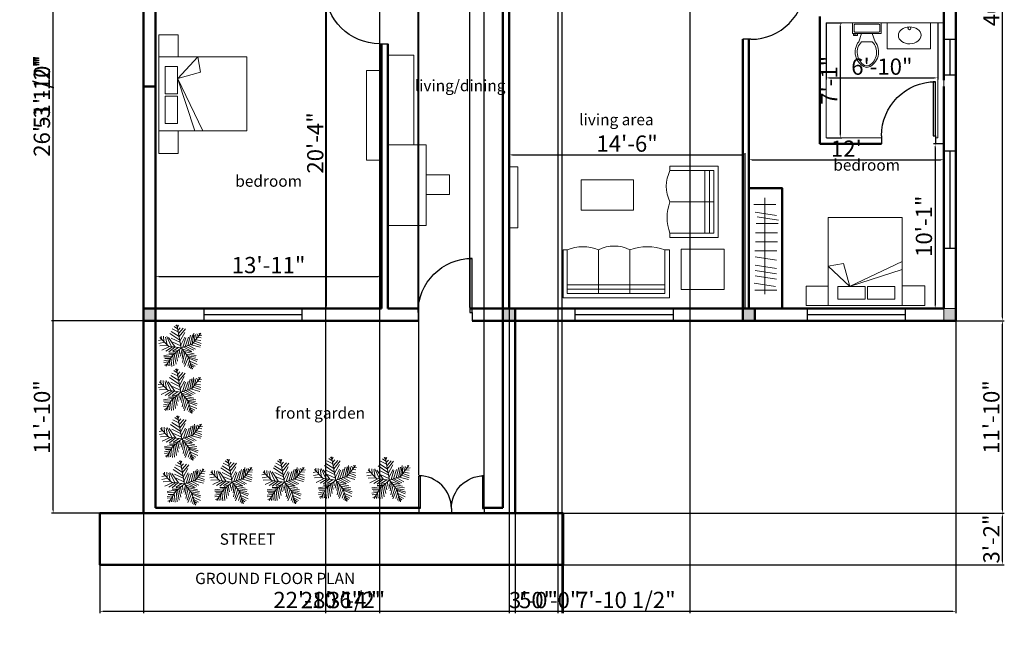
# Model space of a CAD drawing. Units: inches. Extents: x 1367 to 2309, y 1406 to 3826.
# Tile 1 of 9: x 1417 to 2144, y 1406 to 1853. Entities that reach past the tile are written whole.
import ezdxf

# ---------------------------------------------------------------- set-up
doc = ezdxf.new("R2010")
doc.units = ezdxf.units.IN
for name, color, linetype, lineweight in [('A-ANNO-DIMS', 2, 'Continuous', 18), ('A-ANNO-TEXT', 7, 'Continuous', 25), ('A-AREA-IDEN', 3, 'Continuous', 18), ('A-DOOR', 4, 'Continuous', 25), ('A-FLOR-FIXT', 8, 'Continuous', 18), ('A-FURN', 8, 'Continuous', 18), ('A-GLAZ', 4, 'Continuous', 25), ('A-WALL', 7, 'Continuous', 50), ('A-WALL-PATT', 8, 'Continuous', 18), ('garden', 80, 'Continuous', 18)]:
    doc.layers.add(name, color=color, linetype=linetype, lineweight=lineweight)
doc.styles.get("Standard").update_dxf_attribs({"font": 'arial.ttf'})
doc.dimstyles.new('ISO-25', dxfattribs={"dimtxt": 12, "dimasz": 2.5, "dimexe": 1.25, "dimexo": 0.625, "dimtad": 1, "dimdec": 0, "dimlunit": 4, "dimtxsty": 'Standard', "dimcen": 2.5, "dimadec": 0, "dimazin": 0, "dimtfac": 1, "dimtdec": 0, "dimtmove": 0, "dimatfit": 3, "dimfxl": 1, "dimarcsym": 0})

# ---------------------------------------------------------------- blocks, each defined once
blk = doc.blocks.new('*U2')
for p, q in [((0, 0), (0, -6)), ((40, 0), (40, -6))]:
    blk.add_line(p, q)
blk.add_lwpolyline([(0, 0), (0, 40), (1.75, 40), (1.75, 0)], close=True)
blk.add_arc((0, 0), 40, 0, 90)
blk = doc.blocks.new('*U4')
for p, q in [((9.5, -6), (9.5, -2)), ((-10, -8.5), (-8, -8.5)), ((-10, -9.5), (-10, -8.5)), ((-7, -9.5), (-10, -9.5)), ((-8, -8.5), (-8, -8)), ((-7, -8), (-7, -9.5)), ((-4, -8), (-6, -14)), ((4, -14), (-4, -14)), ((4, -8), (6, -14))]:
    blk.add_line(p, q)
blk.add_lwpolyline([(10.5, -8), (10.5, 0), (-10.5, 0), (-10.5, -8)], close=True)
for points in [[(-9.5, -2), (-9.5, -6)], [(8.5, -1), (-8.5, -1)], [(-8.5, -7), (8.5, -7)]]:
    blk.add_lwpolyline(points)
for centre, radius, start, end in [((-8.62, -1.88), 0.884, 81.8699, 188.1301), ((-8.62, -6.12), 0.884, 171.8699, 278.1301), ((8.62, -1.88), 0.884, 351.8699, 98.1301), ((8.62, -6.12), 0.884, 261.8699, 8.1301), ((3.52, -21.58), 12.17, 141.46911, 247.97143), ((4.2, -21.82), 11.33, 136.36773, 238.94682), ((-3.52, -21.58), 12.17, 292.02843, 38.53071), ((-4.2, -21.82), 11.33, 301.05301, 43.63209), ((0, -27.88), 4, 245.73182, 294.26817), ((0, -29), 4, 254.86053, 285.13947)]:
    blk.add_arc(centre, radius, start, end)
blk = doc.blocks.new('*U6')
for p, q in [((-8.737, 47.138), (-17.069, 52.711)), ((-10.186, 53.64), (-13.084, 55.962)), ((0, 0), (-10.5, 57)), ((-9.099, 51.782), (-6.563, 55.962)), ((-7.65, 43.423), (-2.578, 49.46)), ((-31.5, 4.5), (-52.5, 25.5)), ((-48.585, 21.131), (-49.309, 29.026)), ((-43.513, 28.561), (-42.427, 15.558)), ((-38.442, 26.239), (-34.819, 7.663)), ((-35.544, 28.097), (-24.314, 3.947)), ((-14.533, 2.09), (-30.834, 25.31)), ((-3.665, 19.273), (-27.574, 35.527)), ((-5.114, 28.097), (-24.676, 40.636)), ((-7.288, 39.707), (-21.778, 46.673)), ((-5.839, 35.992), (4.667, 48.067)), ((-5.114, 27.632), (10.463, 46.673)), ((-2.941, 16.486), (8.652, 37.85)), ((-1.129, 6.734), (9.014, 26.704)), ((3.942, 1.625), (11.187, 24.381)), ((10.101, 3.483), (17.708, 26.239)), ((16.259, 5.805), (23.142, 31.348)), ((22.055, 7.198), (27.489, 32.277)), ((27, 9), (48, 36)), ((27.127, 9.056), (31.112, 35.992)), ((31.836, 30.883), (32.561, 16.486)), ((35.096, 32.741), (37.27, 22.524)), ((38.719, 34.134), (41.979, 28.561)), ((40.53, 25.775), (48.862, 24.846)), ((43.791, 29.954), (51.036, 30.883)), ((44.153, 36.456), (45.239, 32.741)), ((-47.498, 19.737), (-55.83, 18.344)), ((-40.615, 13.7), (-55.105, 10.913)), ((-33.37, 6.269), (-52.207, 5.34)), ((-28.299, 3.483), (-47.86, -5.805)), ((-21.416, 3.018), (-38.079, -8.128)), ((0, 0), (-31.5, 4.5)), ((-15.982, 2.09), (-30.11, -9.521)), ((-24.314, 23.917), (-2.941, 13.7)), ((0, 0), (-22.5, -19.5)), ((-6.563, 1.161), (-21.416, -8.128)), ((-20.691, 13.7), (-1.129, 4.876)), ((0, 0), (27, 9)), ((0, 0), (18, -22.5)), ((6.478, 1.625), (26.04, -8.592)), ((11.187, 3.483), (30.749, -5.805)), ((18.07, 5.805), (35.096, -3.483)), ((24.229, 7.663), (46.688, 1.625)), ((29.662, 12.307), (48.137, 6.269)), ((33.285, 16.486), (48.862, 10.913)), ((36.183, 19.737), (48.137, 17.88)), ((-17.431, -15.094), (-42.789, -18.809)), ((-24.314, -21.596), (-42.427, -22.06)), ((-22.5, -19.5), (-37.5, -45)), ((-15.257, -12.772), (-30.11, -12.772)), ((-25.038, -23.918), (-22.865, -45.281)), ((-20.691, -18.345), (-17.793, -44.352)), ((-6.563, -5.805), (-19.967, -9.985)), ((-17.069, -15.094), (-12.721, -40.172)), ((-13.446, -11.378), (-8.737, -32.741)), ((-9.461, -8.592), (-6.201, -23.453)), ((-4.752, -3.483), (-3.665, -14.629)), ((2.493, -3.019), (-1.491, -20.202)), ((1.769, -2.555), (24.229, -9.521)), ((5.029, -6.27), (2.131, -25.775)), ((9.014, -11.378), (3.58, -35.992)), ((14.085, -16.951), (6.478, -40.172)), ((7.565, -9.056), (32.198, -14.629)), ((18.07, -22.524), (8.289, -45.745)), ((12.274, -15.094), (36.907, -18.809)), ((16.259, -19.738), (36.183, -22.989)), ((18, -22.5), (27, -52.5)), ((18.433, -22.524), (40.53, -29.026)), ((-28.299, -29.026), (-42.789, -31.348)), ((-30.834, -34.135), (-42.427, -35.528)), ((-34.457, -39.708), (-40.978, -42.494)), ((-26.849, -26.24), (-40.253, -25.775)), ((-32.646, -36.921), (-31.921, -44.352)), ((-29.023, -30.884), (-27.936, -43.887)), ((20.244, -30.419), (15.897, -44.816)), ((19.157, -25.311), (38.719, -33.206)), ((22.78, -37.85), (19.519, -48.532)), ((21.331, -32.741), (39.081, -40.636)), ((22.78, -38.314), (34.372, -44.816)), ((24.591, -45.745), (23.142, -50.854)), ((24.591, -43.423), (30.749, -47.603)), ((26.764, -49.925), (28.213, -50.854))]:
    blk.add_line(p, q)
blk = doc.blocks.new('*D25')
at = {"layer": 'A-ANNO-DIMS', "color": 0, "lineweight": -2, "transparency": 16777216}
for p, q in [((1517.49, 1640.75), (1517.49, 1665.11)), ((1684.37, 1640.75), (1684.37, 1665.11)), ((1519.99, 1663.86), (1681.87, 1663.86))]:
    blk.add_line(p, q, dxfattribs=at)
at = {"layer": 'A-ANNO-DIMS', "color": 0, "lineweight": 100, "transparency": 16777216}
for points in [[(1519.99, 1664.28), (1519.99, 1663.45), (1517.49, 1663.86)], [(1681.87, 1664.28), (1681.87, 1663.45), (1684.37, 1663.86)]]:
    blk.add_solid(points, dxfattribs=at)
at = {"layer": 'Defpoints', "color": 0, "lineweight": 100, "transparency": 16777216}
for p in [(1684.37, 1663.86), (1517.49, 1640.13), (1684.37, 1640.13)]:
    blk.add_point(p, dxfattribs=at)
at = {"layer": 'A-ANNO-DIMS', "color": 0, "transparency": 16777216, "insert": (1600.93, 1670.62), "char_height": 12, "attachment_point": 5}
blk.add_mtext('13\'-11"', dxfattribs=at)
blk = doc.blocks.new('*D26')
at = {"layer": 'A-ANNO-DIMS', "color": 0, "lineweight": -2, "transparency": 16777216}
for p, q in [((1683.74, 1884.56), (1642.43, 1884.56)), ((1643.68, 1642.63), (1643.68, 1882.06)), ((1683.74, 1640.13), (1642.43, 1640.13))]:
    blk.add_line(p, q, dxfattribs=at)
at = {"layer": 'A-ANNO-DIMS', "color": 0, "lineweight": 100, "transparency": 16777216}
for points in [[(1643.26, 1882.06), (1644.09, 1882.06), (1643.68, 1884.56)], [(1643.26, 1642.63), (1644.09, 1642.63), (1643.68, 1640.13)]]:
    blk.add_solid(points, dxfattribs=at)
at = {"layer": 'Defpoints', "color": 0, "lineweight": 100, "transparency": 16777216}
for p in [(1643.68, 1884.56), (1684.37, 1884.56), (1684.37, 1640.13)]:
    blk.add_point(p, dxfattribs=at)
at = {"layer": 'A-ANNO-DIMS', "color": 0, "transparency": 16777216, "insert": (1636.93, 1762.34), "char_height": 12, "attachment_point": 5, "rotation": 90}
blk.add_mtext('20\'-4"', dxfattribs=at)
blk = doc.blocks.new('*D32')
at = {"layer": 'A-ANNO-DIMS', "color": 0, "lineweight": -2, "transparency": 16777216}
for p, q in [((2013.15, 1851.08), (2024.31, 1851.08)), ((2023.06, 1848.58), (2023.06, 1768.57)), ((2013.15, 1766.07), (2024.31, 1766.07))]:
    blk.add_line(p, q, dxfattribs=at)
at = {"layer": 'A-ANNO-DIMS', "color": 0, "lineweight": 100, "transparency": 16777216}
for points in [[(2022.64, 1848.58), (2023.47, 1848.58), (2023.06, 1851.08)], [(2022.64, 1768.57), (2023.47, 1768.57), (2023.06, 1766.07)]]:
    blk.add_solid(points, dxfattribs=at)
at = {"layer": 'Defpoints', "color": 0, "lineweight": 100, "transparency": 16777216}
for p in [(2012.53, 1851.08), (2012.53, 1766.07), (2023.06, 1766.07)]:
    blk.add_point(p, dxfattribs=at)
at = {"layer": 'A-ANNO-DIMS', "color": 0, "transparency": 16777216, "insert": (2016.41, 1808.58), "char_height": 12, "attachment_point": 5, "rotation": 90}
blk.add_mtext('7\'-1"', dxfattribs=at)
blk = doc.blocks.new('*D33')
at = {"layer": 'A-ANNO-DIMS', "color": 0, "lineweight": -2, "transparency": 16777216}
for p, q in [((2012.53, 1850.45), (2012.53, 1809.12)), ((2094.99, 1850.45), (2094.99, 1809.12)), ((2015.03, 1810.37), (2092.49, 1810.37))]:
    blk.add_line(p, q, dxfattribs=at)
at = {"layer": 'A-ANNO-DIMS', "color": 0, "lineweight": 100, "transparency": 16777216}
for points in [[(2015.03, 1810.79), (2015.03, 1809.95), (2012.53, 1810.37)], [(2092.49, 1810.79), (2092.49, 1809.95), (2094.99, 1810.37)]]:
    blk.add_solid(points, dxfattribs=at)
at = {"layer": 'Defpoints', "color": 0, "lineweight": 100, "transparency": 16777216}
for p in [(2012.53, 1851.08), (2094.99, 1851.08), (2094.99, 1810.37)]:
    blk.add_point(p, dxfattribs=at)
at = {"layer": 'A-ANNO-DIMS', "color": 0, "transparency": 16777216, "insert": (2053.76, 1817.12), "char_height": 12, "attachment_point": 5}
blk.add_mtext('6\'-10"', dxfattribs=at)
blk = doc.blocks.new('*D34')
at = {"layer": 'A-ANNO-DIMS', "color": 0, "lineweight": -2, "transparency": 16777216}
for p, q in [((1955.49, 1640.75), (1955.49, 1751.18)), ((1957.99, 1749.93), (2096.99, 1749.93)), ((2099.49, 1640.75), (2099.49, 1751.18))]:
    blk.add_line(p, q, dxfattribs=at)
at = {"layer": 'A-ANNO-DIMS', "color": 0, "lineweight": 100, "transparency": 16777216}
for points in [[(1957.99, 1750.35), (1957.99, 1749.51), (1955.49, 1749.93)], [(2096.99, 1750.35), (2096.99, 1749.51), (2099.49, 1749.93)]]:
    blk.add_solid(points, dxfattribs=at)
at = {"layer": 'Defpoints', "color": 0, "lineweight": 100, "transparency": 16777216}
for p in [(2099.49, 1749.93), (1955.49, 1640.13), (2099.49, 1640.13)]:
    blk.add_point(p, dxfattribs=at)
at = {"layer": 'A-ANNO-DIMS', "color": 0, "transparency": 16777216, "insert": (2027.49, 1756.58), "char_height": 12, "attachment_point": 5}
blk.add_mtext("12'", dxfattribs=at)
blk = doc.blocks.new('*D35')
at = {"layer": 'A-ANNO-DIMS', "color": 0, "lineweight": -2, "transparency": 16777216}
for p, q in [((2098.87, 1761.57), (2091.88, 1761.57)), ((2093.13, 1759.07), (2093.13, 1642.63)), ((2098.87, 1640.13), (2091.88, 1640.13))]:
    blk.add_line(p, q, dxfattribs=at)
at = {"layer": 'A-ANNO-DIMS', "color": 0, "lineweight": 100, "transparency": 16777216}
for points in [[(2092.72, 1759.07), (2093.55, 1759.07), (2093.13, 1761.57)], [(2092.72, 1642.63), (2093.55, 1642.63), (2093.13, 1640.13)]]:
    blk.add_solid(points, dxfattribs=at)
at = {"layer": 'Defpoints', "color": 0, "lineweight": 100, "transparency": 16777216}
for p in [(2099.49, 1761.57), (2093.13, 1640.13), (2099.49, 1640.13)]:
    blk.add_point(p, dxfattribs=at)
at = {"layer": 'A-ANNO-DIMS', "color": 0, "transparency": 16777216, "insert": (2086.38, 1700.85), "char_height": 12, "attachment_point": 5, "rotation": 90}
blk.add_mtext('10\'-1"', dxfattribs=at)
blk = doc.blocks.new('*D36')
at = {"layer": 'A-ANNO-DIMS', "color": 0, "lineweight": -2, "transparency": 16777216}
for p, q in [((1778.49, 1640.75), (1778.49, 1754.79)), ((1780.99, 1753.54), (1950.3, 1753.54)), ((1952.8, 1640.75), (1952.8, 1754.79))]:
    blk.add_line(p, q, dxfattribs=at)
at = {"layer": 'A-ANNO-DIMS', "color": 0, "lineweight": 100, "transparency": 16777216}
for points in [[(1780.99, 1753.96), (1780.99, 1753.13), (1778.49, 1753.54)], [(1950.3, 1753.96), (1950.3, 1753.13), (1952.8, 1753.54)]]:
    blk.add_solid(points, dxfattribs=at)
at = {"layer": 'Defpoints', "color": 0, "lineweight": 100, "transparency": 16777216}
for p in [(1952.8, 1753.54), (1778.49, 1640.13), (1952.8, 1640.13)]:
    blk.add_point(p, dxfattribs=at)
at = {"layer": 'A-ANNO-DIMS', "color": 0, "transparency": 16777216, "insert": (1865.65, 1760.3), "char_height": 12, "attachment_point": 5}
blk.add_mtext('14\'-6"', dxfattribs=at)
blk = doc.blocks.new('SOFA-3')
for p, q in [((3.39, 35.52), (0, 35.52)), ((0, 35.52), (0, 0)), ((29.28, 35.52), (29.28, 3.13)), ((52.37, 35.52), (52.37, 3.13)), ((75.45, 35.52), (78.61, 35.52)), ((78.61, 0), (78.61, 35.52)), ((0, 0), (78.61, 0))]:
    blk.add_line(p, q)
blk.add_lwpolyline([(3.39, 35.52), (3.39, 3.13), (75.45, 3.13), (75.45, 35.52)])
for centre, radius, start, end in [((16.33, -1.36), 39.09, 70.66096, 109.33904), ((40.82, 12.11), 26.1, 63.74962, 116.25038), ((63.91, 5.49), 32.17, 68.97185, 111.02815)]:
    blk.add_arc(centre, radius, start, end)
blk = doc.blocks.new('ARMCHAIR')
for p, q in [((0, 52.73), (0, 0)), ((35.52, 52.73), (0, 52.73)), ((35.52, 49.34), (35.52, 52.73)), ((35.52, 49.34), (3.13, 49.34)), ((35.52, 26.25), (3.13, 26.25)), ((35.52, 3.16), (35.52, 0)), ((0, 0), (35.52, 0))]:
    blk.add_line(p, q)
blk.add_lwpolyline([(3.13, 49.34), (3.13, 3.16), (35.52, 3.16)])
for centre, radius, start, end in [((12.11, 37.79), 26.1, 333.74962, 26.25038), ((5.49, 14.7), 32.17, 338.97185, 21.02815)]:
    blk.add_arc(centre, radius, start, end)
blk = doc.blocks.new('*D55')
at = {"layer": 'A-ANNO-DIMS', "color": 0, "lineweight": -2, "transparency": 16777216}
for p, q in [((1508.49, 1630.5), (1508.49, 1415.33)), ((2108.49, 1630.5), (2108.49, 1415.33)), ((1510.99, 1416.58), (2105.99, 1416.58))]:
    blk.add_line(p, q, dxfattribs=at)
at = {"layer": 'A-ANNO-DIMS', "color": 0, "lineweight": 100, "transparency": 16777216}
for points in [[(1510.99, 1416.99), (1510.99, 1416.16), (1508.49, 1416.58)], [(2105.99, 1416.99), (2105.99, 1416.16), (2108.49, 1416.58)]]:
    blk.add_solid(points, dxfattribs=at)
at = {"layer": 'Defpoints', "color": 0, "lineweight": 100, "transparency": 16777216}
for p in [(1508.49, 1631.13), (2108.49, 1631.13), (2108.49, 1416.58)]:
    blk.add_point(p, dxfattribs=at)
at = {"layer": 'A-ANNO-DIMS', "color": 0, "transparency": 16777216, "insert": (1808.49, 1423.33), "char_height": 12, "attachment_point": 5}
blk.add_mtext('50\'-0"', dxfattribs=at)
blk = doc.blocks.new('*D56')
at = {"layer": 'A-ANNO-DIMS', "color": 0, "lineweight": -2, "transparency": 16777216}
for p, q in [((1508.49, 1630.5), (1508.49, 1415.33)), ((1782.99, 1630.5), (1782.99, 1415.33)), ((1510.99, 1416.58), (1780.49, 1416.58))]:
    blk.add_line(p, q, dxfattribs=at)
at = {"layer": 'A-ANNO-DIMS', "color": 0, "lineweight": 100, "transparency": 16777216}
for points in [[(1510.99, 1416.99), (1510.99, 1416.16), (1508.49, 1416.58)], [(1780.49, 1416.99), (1780.49, 1416.16), (1782.99, 1416.58)]]:
    blk.add_solid(points, dxfattribs=at)
at = {"layer": 'Defpoints', "color": 0, "lineweight": 100, "transparency": 16777216}
for p in [(1508.49, 1631.13), (1782.99, 1631.13), (1782.99, 1416.58)]:
    blk.add_point(p, dxfattribs=at)
at = {"layer": 'A-ANNO-DIMS', "color": 0, "transparency": 16777216, "insert": (1645.74, 1423.41), "char_height": 12, "attachment_point": 5}
blk.add_mtext('22\'-10 1/2"', dxfattribs=at)
blk = doc.blocks.new('*D67')
at = {"layer": 'A-ANNO-DIMS', "color": 0, "lineweight": -2, "transparency": 16777216}
for p, q in [((2109.15, 2111.13), (2144.18, 2111.13)), ((2142.93, 1633.63), (2142.93, 2108.63)), ((2109.12, 1631.13), (2144.18, 1631.13))]:
    blk.add_line(p, q, dxfattribs=at)
at = {"layer": 'A-ANNO-DIMS', "color": 0, "lineweight": 100, "transparency": 16777216}
for points in [[(2142.51, 2108.63), (2143.34, 2108.63), (2142.93, 2111.13)], [(2142.51, 1633.63), (2143.34, 1633.63), (2142.93, 1631.13)]]:
    blk.add_solid(points, dxfattribs=at)
at = {"layer": 'Defpoints', "color": 0, "lineweight": 100, "transparency": 16777216}
for p in [(2108.53, 2111.13), (2142.93, 2111.13), (2108.49, 1631.13)]:
    blk.add_point(p, dxfattribs=at)
at = {"layer": 'A-ANNO-DIMS', "color": 0, "transparency": 16777216, "insert": (2136.17, 1871.13), "char_height": 12, "attachment_point": 5, "rotation": 90}
blk.add_mtext('40\'-0"', dxfattribs=at)
blk = doc.blocks.new('*D68')
at = {"layer": 'A-ANNO-DIMS', "color": 0, "lineweight": -2, "transparency": 16777216}
for p, q in [((1819.04, 1488.94), (2144.18, 1488.94)), ((2142.93, 1453.48), (2142.93, 1486.44)), ((1819.04, 1450.98), (2144.18, 1450.98))]:
    blk.add_line(p, q, dxfattribs=at)
at = {"layer": 'A-ANNO-DIMS', "color": 0, "lineweight": 100, "transparency": 16777216}
for points in [[(2142.51, 1486.44), (2143.34, 1486.44), (2142.93, 1488.94)], [(2142.51, 1453.48), (2143.34, 1453.48), (2142.93, 1450.98)]]:
    blk.add_solid(points, dxfattribs=at)
at = {"layer": 'Defpoints', "color": 0, "lineweight": 100, "transparency": 16777216}
for p in [(1818.41, 1488.94), (2142.93, 1488.94), (1818.41, 1450.98)]:
    blk.add_point(p, dxfattribs=at)
at = {"layer": 'A-ANNO-DIMS', "color": 0, "transparency": 16777216, "insert": (2136.17, 1469.96), "char_height": 12, "attachment_point": 5, "rotation": 90}
blk.add_mtext('3\'-2"', dxfattribs=at)
blk = doc.blocks.new('*D69')
at = {"layer": 'A-ANNO-DIMS', "color": 0, "lineweight": -2, "transparency": 16777216}
for p, q in [((1783.62, 1631.13), (2144.18, 1631.13)), ((2142.93, 1491.44), (2142.93, 1628.63)), ((1783.62, 1488.94), (2144.18, 1488.94))]:
    blk.add_line(p, q, dxfattribs=at)
at = {"layer": 'A-ANNO-DIMS', "color": 0, "lineweight": 100, "transparency": 16777216}
for points in [[(2142.51, 1628.63), (2143.34, 1628.63), (2142.93, 1631.13)], [(2142.51, 1491.44), (2143.34, 1491.44), (2142.93, 1488.94)]]:
    blk.add_solid(points, dxfattribs=at)
at = {"layer": 'Defpoints', "color": 0, "lineweight": 100, "transparency": 16777216}
for p in [(1782.99, 1631.13), (2142.93, 1631.13), (1782.99, 1488.94)]:
    blk.add_point(p, dxfattribs=at)
at = {"layer": 'A-ANNO-DIMS', "color": 0, "transparency": 16777216, "insert": (2136.17, 1560.03), "char_height": 12, "attachment_point": 5, "rotation": 90}
blk.add_mtext('11\'-10"', dxfattribs=at)
blk = doc.blocks.new('*D70')
at = {"layer": 'A-ANNO-DIMS', "color": 0, "lineweight": -2, "transparency": 16777216}
for p, q in [((1507.87, 2111.13), (1440.62, 2111.13)), ((1441.87, 1491.44), (1441.87, 2108.63)), ((1507.87, 1488.94), (1440.62, 1488.94))]:
    blk.add_line(p, q, dxfattribs=at)
at = {"layer": 'A-ANNO-DIMS', "color": 0, "lineweight": 100, "transparency": 16777216}
for points in [[(1441.45, 2108.63), (1442.28, 2108.63), (1441.87, 2111.13)], [(1441.45, 1491.44), (1442.28, 1491.44), (1441.87, 1488.94)]]:
    blk.add_solid(points, dxfattribs=at)
at = {"layer": 'Defpoints', "color": 0, "lineweight": 100, "transparency": 16777216}
for p in [(1441.87, 2111.13), (1508.49, 2111.13), (1508.49, 1488.94)]:
    blk.add_point(p, dxfattribs=at)
at = {"layer": 'A-ANNO-DIMS', "color": 0, "transparency": 16777216, "insert": (1435.11, 1800.03), "char_height": 12, "attachment_point": 5, "rotation": 90}
blk.add_mtext('51\'-10"', dxfattribs=at)
blk = doc.blocks.new('*D71')
at = {"layer": 'A-ANNO-DIMS', "color": 0, "lineweight": -2, "transparency": 16777216}
for p, q in [((1507.87, 1631.13), (1440.62, 1631.13)), ((1441.87, 1491.44), (1441.87, 1628.63)), ((1507.87, 1488.94), (1440.62, 1488.94))]:
    blk.add_line(p, q, dxfattribs=at)
at = {"layer": 'A-ANNO-DIMS', "color": 0, "lineweight": 100, "transparency": 16777216}
for points in [[(1441.45, 1628.63), (1442.28, 1628.63), (1441.87, 1631.13)], [(1441.45, 1491.44), (1442.28, 1491.44), (1441.87, 1488.94)]]:
    blk.add_solid(points, dxfattribs=at)
at = {"layer": 'Defpoints', "color": 0, "lineweight": 100, "transparency": 16777216}
for p in [(1441.87, 1631.13), (1508.49, 1631.13), (1508.49, 1488.94)]:
    blk.add_point(p, dxfattribs=at)
at = {"layer": 'A-ANNO-DIMS', "color": 0, "transparency": 16777216, "insert": (1435.11, 1560.03), "char_height": 12, "attachment_point": 5, "rotation": 90}
blk.add_mtext('11\'-10"', dxfattribs=at)
blk = doc.blocks.new('*D72')
at = {"layer": 'A-ANNO-DIMS', "color": 0, "lineweight": -2, "transparency": 16777216}
for p, q in [((1507.87, 1946.63), (1440.62, 1946.63)), ((1441.87, 1633.63), (1441.87, 1944.13)), ((1507.87, 1631.13), (1440.62, 1631.13))]:
    blk.add_line(p, q, dxfattribs=at)
at = {"layer": 'A-ANNO-DIMS', "color": 0, "lineweight": 100, "transparency": 16777216}
for points in [[(1441.45, 1944.13), (1442.28, 1944.13), (1441.87, 1946.63)], [(1441.45, 1633.63), (1442.28, 1633.63), (1441.87, 1631.13)]]:
    blk.add_solid(points, dxfattribs=at)
at = {"layer": 'Defpoints', "color": 0, "lineweight": 100, "transparency": 16777216}
for p in [(1441.87, 1946.63), (1508.49, 1946.63), (1508.49, 1631.13)]:
    blk.add_point(p, dxfattribs=at)
at = {"layer": 'A-ANNO-DIMS', "color": 0, "transparency": 16777216, "insert": (1435.03, 1788.88), "char_height": 12, "attachment_point": 5, "rotation": 90}
blk.add_mtext('26\'-3 1/2"', dxfattribs=at)
blk = doc.blocks.new('*D75')
at = {"layer": 'A-ANNO-DIMS', "color": 0, "lineweight": -2, "transparency": 16777216}
for p, q in [((1476.27, 1450.35), (1476.27, 1415.33)), ((1818.41, 1450.35), (1818.41, 1415.33)), ((1478.77, 1416.58), (1815.91, 1416.58))]:
    blk.add_line(p, q, dxfattribs=at)
at = {"layer": 'A-ANNO-DIMS', "color": 0, "lineweight": 100, "transparency": 16777216}
for points in [[(1478.77, 1416.99), (1478.77, 1416.16), (1476.27, 1416.58)], [(1815.91, 1416.99), (1815.91, 1416.16), (1818.41, 1416.58)]]:
    blk.add_solid(points, dxfattribs=at)
at = {"layer": 'Defpoints', "color": 0, "lineweight": 100, "transparency": 16777216}
for p in [(1476.27, 1450.98), (1818.41, 1450.98), (1818.41, 1416.58)]:
    blk.add_point(p, dxfattribs=at)
at = {"layer": 'A-ANNO-DIMS', "color": 0, "transparency": 16777216, "insert": (1647.34, 1423.33), "char_height": 12, "attachment_point": 5}
blk.add_mtext('28\'-6"', dxfattribs=at)
blk = doc.blocks.new('*D76')
at = {"layer": 'A-ANNO-DIMS', "color": 0, "lineweight": -2, "transparency": 16777216}
for p, q in [((1711.82, 1517.28), (1711.82, 2146.78)), ((1714.32, 2145.53), (1757.51, 2145.53)), ((1760.01, 1517.28), (1760.01, 2146.78))]:
    blk.add_line(p, q, dxfattribs=at)
at = {"layer": 'A-ANNO-DIMS', "color": 0, "lineweight": 100, "transparency": 16777216}
for points in [[(1714.32, 2145.94), (1714.32, 2145.11), (1711.82, 2145.53)], [(1757.51, 2145.94), (1757.51, 2145.11), (1760.01, 2145.53)]]:
    blk.add_solid(points, dxfattribs=at)
at = {"layer": 'Defpoints', "color": 0, "lineweight": 100, "transparency": 16777216}
for p in [(1760.01, 2145.53), (1711.82, 1516.65), (1760.01, 1516.65)]:
    blk.add_point(p, dxfattribs=at)
at = {"layer": 'A-ANNO-DIMS', "color": 0, "transparency": 16777216, "insert": (1735.92, 2152.28), "char_height": 12, "attachment_point": 5}
blk.add_mtext('4\'-0"', dxfattribs=at)
blk = doc.blocks.new('*D77')
at = {"layer": 'A-ANNO-DIMS', "color": 0, "lineweight": -2, "transparency": 16777216}
for p, q in [((1760.01, 1493.18), (1760.01, 2146.78)), ((1762.51, 2145.53), (1771.49, 2145.53)), ((1773.99, 1493.56), (1773.99, 2146.78)), ((1773.99, 2145.53), (1808.51, 2145.53))]:
    blk.add_line(p, q, dxfattribs=at)
at = {"layer": 'A-ANNO-DIMS', "color": 0, "lineweight": 100, "transparency": 16777216}
for points in [[(1762.51, 2145.94), (1762.51, 2145.11), (1760.01, 2145.53)], [(1771.49, 2145.94), (1771.49, 2145.11), (1773.99, 2145.53)]]:
    blk.add_solid(points, dxfattribs=at)
at = {"layer": 'Defpoints', "color": 0, "lineweight": 100, "transparency": 16777216}
for p in [(1773.99, 2145.53), (1760.01, 1492.55), (1773.99, 1492.94)]:
    blk.add_point(p, dxfattribs=at)
at = {"layer": 'A-ANNO-DIMS', "color": 0, "transparency": 16777216, "insert": (1792.5, 2152.18), "char_height": 12, "attachment_point": 5}
blk.add_mtext('1\'-2"', dxfattribs=at)
blk = doc.blocks.new('*D78')
at = {"layer": 'A-ANNO-DIMS', "color": 0, "lineweight": -2, "transparency": 16777216}
for p, q in [((1711.4, 1640.75), (1711.4, 2146.78)), ((1713.9, 2145.53), (1747.03, 2145.53)), ((1749.53, 1640.75), (1749.53, 2146.78))]:
    blk.add_line(p, q, dxfattribs=at)
at = {"layer": 'A-ANNO-DIMS', "color": 0, "lineweight": 100, "transparency": 16777216}
for points in [[(1713.9, 2145.94), (1713.9, 2145.11), (1711.4, 2145.53)], [(1747.03, 2145.94), (1747.03, 2145.11), (1749.53, 2145.53)]]:
    blk.add_solid(points, dxfattribs=at)
at = {"layer": 'Defpoints', "color": 0, "lineweight": 100, "transparency": 16777216}
for p in [(1749.53, 2145.53), (1711.4, 1640.13), (1749.53, 1640.13)]:
    blk.add_point(p, dxfattribs=at)
at = {"layer": 'A-ANNO-DIMS', "color": 0, "transparency": 16777216, "insert": (1730.47, 2152.28), "char_height": 12, "attachment_point": 5}
blk.add_mtext('3\'-2"', dxfattribs=at)
blk = doc.blocks.new('*D79')
at = {"layer": 'A-ANNO-DIMS', "color": 0, "lineweight": -2, "transparency": 16777216}
for p, q in [((1778.49, 1990.06), (1778.49, 1415.33)), ((1814.49, 1990.06), (1814.49, 1415.33)), ((1780.99, 1416.58), (1811.99, 1416.58))]:
    blk.add_line(p, q, dxfattribs=at)
at = {"layer": 'A-ANNO-DIMS', "color": 0, "lineweight": 100, "transparency": 16777216}
for points in [[(1780.99, 1416.99), (1780.99, 1416.16), (1778.49, 1416.58)], [(1811.99, 1416.99), (1811.99, 1416.16), (1814.49, 1416.58)]]:
    blk.add_solid(points, dxfattribs=at)
at = {"layer": 'Defpoints', "color": 0, "lineweight": 100, "transparency": 16777216}
for p in [(1778.49, 1990.68), (1814.49, 1990.68), (1814.49, 1416.58)]:
    blk.add_point(p, dxfattribs=at)
at = {"layer": 'A-ANNO-DIMS', "color": 0, "transparency": 16777216, "insert": (1796.49, 1423.33), "char_height": 12, "attachment_point": 5}
blk.add_mtext('3\'-0"', dxfattribs=at)
blk = doc.blocks.new('*D80')
at = {"layer": 'A-ANNO-DIMS', "color": 0, "lineweight": -2, "transparency": 16777216}
for p, q in [((1817.49, 1993.06), (1817.49, 1415.33)), ((1911.99, 1993.06), (1911.99, 1415.33)), ((1819.99, 1416.58), (1909.49, 1416.58))]:
    blk.add_line(p, q, dxfattribs=at)
at = {"layer": 'A-ANNO-DIMS', "color": 0, "lineweight": 100, "transparency": 16777216}
for points in [[(1819.99, 1416.99), (1819.99, 1416.16), (1817.49, 1416.58)], [(1909.49, 1416.99), (1909.49, 1416.16), (1911.99, 1416.58)]]:
    blk.add_solid(points, dxfattribs=at)
at = {"layer": 'Defpoints', "color": 0, "lineweight": 100, "transparency": 16777216}
for p in [(1817.49, 1993.68), (1911.99, 1993.68), (1911.99, 1416.58)]:
    blk.add_point(p, dxfattribs=at)
at = {"layer": 'A-ANNO-DIMS', "color": 0, "transparency": 16777216, "insert": (1864.74, 1423.41), "char_height": 12, "attachment_point": 5}
blk.add_mtext('7\'-10 1/2"', dxfattribs=at)
blk = doc.blocks.new('*D136')
at = {"layer": 'A-ANNO-DIMS', "color": 0, "lineweight": -2, "transparency": 16777216}
for p, q in [((1642.87, 1897.66), (1642.87, 1415.33)), ((1682.87, 1897.66), (1682.87, 1415.33)), ((1645.37, 1416.58), (1680.37, 1416.58))]:
    blk.add_line(p, q, dxfattribs=at)
at = {"layer": 'A-ANNO-DIMS', "color": 0, "lineweight": 100, "transparency": 16777216}
for points in [[(1645.37, 1416.99), (1645.37, 1416.16), (1642.87, 1416.58)], [(1680.37, 1416.99), (1680.37, 1416.16), (1682.87, 1416.58)]]:
    blk.add_solid(points, dxfattribs=at)
at = {"layer": 'Defpoints', "color": 0, "lineweight": 100, "transparency": 16777216}
for p in [(1642.87, 1898.28), (1682.87, 1898.28), (1682.87, 1416.58)]:
    blk.add_point(p, dxfattribs=at)
at = {"layer": 'A-ANNO-DIMS', "color": 0, "transparency": 16777216, "insert": (1662.87, 1423.33), "char_height": 12, "attachment_point": 5}
blk.add_mtext('3\'-4"', dxfattribs=at)

msp = doc.modelspace()

# ---------------------------------------------------------------- hatches: boundary and pattern name
at = {"layer": 'A-WALL-PATT'}
h = msp.add_hatch(color=256, dxfattribs=at)
h.dxf.hatch_style = 1
h.paths.add_polyline_path([(1508.49, 1631.13), (1517.49, 1631.13), (1517.49, 1640.13), (1508.49, 1640.13)])
h.paths.add_polyline_path([(1773.99, 1631.13), (1782.99, 1631.13), (1782.99, 1640.13), (1773.99, 1640.13)])
h.paths.add_polyline_path([(1959.99, 1631.13), (1959.99, 1640.13), (1950.99, 1640.13), (1950.99, 1631.13)])
h.paths.add_polyline_path([(2099.49, 1640.13), (2099.49, 1631.13), (2108.49, 1631.13), (2108.49, 1640.13)])
h.paths.add_polyline_path([(1706.06, 1795.81), (1771.22, 1795.81), (1771.22, 1813.02), (1706.06, 1813.02)], flags=9)
h.paths.add_polyline_path([(1573.51, 1725.43), (1623.74, 1725.43), (1623.74, 1742.65), (1573.51, 1742.65)], flags=9)
h.paths.add_polyline_path([(1582.26, 2004.3), (1623.41, 2004.3), (1623.41, 2021.52), (1582.26, 2021.52)], flags=9)
h.paths.add_polyline_path([(1992.39, 1973.53), (2042.62, 1973.53), (2042.62, 1990.75), (1992.39, 1990.75)], flags=9)
h.paths.add_polyline_path([(2015.09, 1737.31), (2065.32, 1737.31), (2065.32, 1754.53), (2015.09, 1754.53)], flags=9)
h.paths.add_polyline_path([(1827.45, 1770.85), (1884.81, 1770.85), (1884.81, 1788.06), (1827.45, 1788.06)], flags=9)

# ---------------------------------------------------------------- linework, layer by layer
at = {"layer": 'A-FURN'}
for p, q in [((2096.58, 1851.08), (2012.53, 1851.08)), ((2012.53, 1851.08), (2094.99, 1851.08)), ((2012.53, 1851.08), (2012.53, 1766.07)), ((2089.77, 1851.08), (2089.77, 1831.73)), ((2094.99, 1766.07), (2094.99, 1851.08)), ((2096.58, 1851.08), (2099.49, 1851.08)), ((2099.49, 1765.68), (2099.49, 1851.08)), ((1533.81, 1809.84), (1548.67, 1825.92)), ((1548.67, 1825.92), (1550.62, 1814.7)), ((2099.49, 1826.56), (2099.49, 1831.06)), ((1550.62, 1814.7), (1533.81, 1809.84)), ((1950.99, 1814.85), (1950.99, 1799.12)), ((1955.49, 1814.85), (1955.49, 1808.62)), ((1955.49, 1814.85), (1955.49, 1799.12)), ((1533.65, 1810.18), (1546.37, 1771.36)), ((1533.65, 1810.18), (1552.28, 1771.36)), ((1955.49, 1804.12), (1955.49, 1799.12)), ((2053.46, 1766.07), (2012.53, 1766.07)), ((2094.99, 1766.07), (2093.46, 1766.07)), ((2099.49, 1761.57), (2093.46, 1761.57)), ((2099.49, 1766.07), (2099.49, 1761.57)), ((1923.13, 1741.91), (1923.13, 1695.74)), ((1926.48, 1741.91), (1926.48, 1695.74)), ((1975.53, 1716.97), (1959.21, 1716.97)), ((1967.37, 1650.68), (1967.37, 1721.94)), ((1975.99, 1708.81), (1960.33, 1711.26)), ((1977.27, 1702.9), (1960.95, 1702.9)), ((1977.4, 1705.35), (1961.73, 1707.8)), ((1976.81, 1695.97), (1960.49, 1695.97)), ((1976.81, 1689.28), (1960.49, 1689.28)), ((1976.3, 1682.59), (1959.98, 1682.59)), ((1975.99, 1675.7), (1960.33, 1678.15)), ((2014.14, 1671.3), (2025.36, 1673.25)), ((2025.36, 1673.25), (2030.22, 1656.45)), ((2029.88, 1656.28), (2068.69, 1674.92)), ((1975.99, 1669.56), (1960.33, 1672.02)), ((1975.99, 1665.68), (1960.33, 1668.14)), ((2030.22, 1656.45), (2014.14, 1671.3)), ((2029.88, 1656.28), (2068.69, 1669)), ((1893.54, 1657.7), (1821.47, 1657.7)), ((1975.14, 1656.48), (1959.48, 1658.93)), ((1975.99, 1661.8), (1960.33, 1664.26)), ((1893.54, 1654.35), (1821.47, 1654.35)), ((1976.3, 1653.59), (1959.98, 1653.59)), ((1962.73, 1653.59), (1976.3, 1653.59)), ((1735.91, 1492.94), (1735.92, 1492.94))]:
    msp.add_line(p, q, dxfattribs=at)
for points in [[(2089.77, 1831.73), (2089.77, 1851.08), (2057.6, 1851.08), (2057.6, 1831.73)], [(1519.81, 1825.92), (1519.81, 1842.19), (1534.08, 1842.19), (1534.08, 1825.92)], [(1519.81, 1771.36), (1519.81, 1825.92), (1584.75, 1825.92), (1584.75, 1771.36)], [(1688.87, 1827.23), (1708.16, 1827.23), (1708.16, 1760.99), (1688.87, 1760.99)], [(1524.44, 1798.6), (1524.44, 1818.79), (1533.65, 1818.79), (1533.65, 1798.6)], [(1684.37, 1815.73), (1673.11, 1815.73), (1673.11, 1749.67), (1684.37, 1749.67)], [(1524.44, 1776.73), (1524.44, 1796.92), (1533.65, 1796.92), (1533.65, 1776.73)], [(1519.81, 1771.36), (1519.81, 1754.54), (1534.22, 1754.54), (1534.22, 1771.36)], [(1688.87, 1760.99), (1717.18, 1760.99), (1717.18, 1701.5), (1688.87, 1701.5)], [(1717.18, 1738.78), (1734.4, 1738.78), (1734.4, 1724.4), (1717.18, 1724.4)], [(1778.49, 1744.6), (1784.86, 1744.6), (1784.86, 1699.62), (1778.49, 1699.62)], [(1870.44, 1735.15), (1831.63, 1735.15), (1831.63, 1712.83), (1870.44, 1712.83)], [(2068.69, 1642.45), (2014.14, 1642.45), (2014.14, 1707.39), (2068.69, 1707.39)], [(1937.38, 1654.18), (1905.67, 1654.18), (1905.67, 1684.01), (1937.38, 1684.01)], [(2014.14, 1642.45), (1997.87, 1642.45), (1997.87, 1656.71), (2014.14, 1656.71)], [(2041.45, 1647.08), (2021.26, 1647.08), (2021.26, 1656.28), (2041.45, 1656.28)], [(2063.33, 1647.08), (2043.14, 1647.08), (2043.14, 1656.28), (2063.33, 1656.28)], [(2068.69, 1642.45), (2085.51, 1642.45), (2085.51, 1656.85), (2068.69, 1656.85)], [(2099.49, 1640.13), (2108.49, 1640.13), (2108.49, 1631.13), (2099.49, 1631.13)]]:
    msp.add_lwpolyline(points, close=True, dxfattribs=at)
msp.add_circle((2074.07, 1846.98), 1.06, dxfattribs=at)
msp.add_ellipse((2074.33, 1841.76), major_axis=(-8.38, -0.17), ratio=0.747916, dxfattribs=at)
at = {"layer": 'A-GLAZ'}
for p, q in [((2103.99, 1838.77), (2103.99, 1812.7)), ((2103.99, 1756.53), (2103.99, 1684.37)), ((1553.28, 1635.63), (1625.44, 1635.63)), ((1827.38, 1635.63), (1899.54, 1635.63)), ((1998.79, 1635.63), (2070.95, 1635.63))]:
    msp.add_line(p, q, dxfattribs=at)
for points in [[(2099.49, 1838.77), (2099.49, 1812.7), (2108.49, 1812.7), (2108.49, 1838.77)], [(2108.49, 1756.53), (2108.49, 1684.37), (2099.49, 1684.37), (2099.49, 1756.53)], [(1553.28, 1640.13), (1625.44, 1640.13), (1625.44, 1631.13), (1553.28, 1631.13)], [(1827.38, 1640.13), (1899.54, 1640.13), (1899.54, 1631.13), (1827.38, 1631.13)], [(1998.79, 1640.13), (2070.95, 1640.13), (2070.95, 1631.13), (1998.79, 1631.13)]]:
    msp.add_lwpolyline(points, close=True, dxfattribs=at)
at = {"layer": 'A-WALL'}
for p, q in [((1773.99, 1759.12), (1773.99, 1947.33)), ((1778.49, 1759.12), (1778.49, 1947.33)), ((2008.03, 1855.58), (2008.03, 1851.08)), ((2008.03, 1851.08), (2008.03, 1761.57)), ((1684.37, 1835.57), (1684.37, 1640.13)), ((1688.87, 1835.57), (1688.87, 1640.13)), ((1950.99, 1759.12), (1950.99, 1838.85)), ((1955.49, 1759.12), (1955.49, 1838.85)), ((1517.49, 1804.12), (1508.49, 1804.12)), ((1517.49, 1804.12), (1517.49, 1640.13)), ((2053.46, 1761.57), (2008.03, 1761.57)), ((1773.99, 1759.12), (1773.99, 1640.13)), ((1778.49, 1759.12), (1778.49, 1640.13)), ((1950.99, 1759.12), (1950.99, 1640.13)), ((1955.49, 1759.12), (1955.49, 1640.13)), ((1601.49, 1640.13), (1517.49, 1640.13)), ((1653.99, 1640.13), (1601.49, 1640.13)), ((1601.49, 1640.13), (1605.99, 1640.13)), ((1684.37, 1640.13), (1653.99, 1640.13)), ((1711.4, 1640.13), (1688.87, 1640.13)), ((1773.99, 1640.13), (1749.53, 1640.13)), ((1508.49, 1631.13), (1508.49, 1488.94)), ((1517.49, 1631.13), (1517.49, 1492.94)), ((1773.99, 1631.13), (1773.99, 1492.94)), ((1782.99, 1631.13), (1782.99, 1488.94)), ((1517.49, 1492.94), (1712.87, 1492.94)), ((1758.96, 1492.94), (1773.99, 1492.94)), ((1508.49, 1488.94), (1711.82, 1488.94)), ((1760.01, 1488.94), (1782.99, 1488.94))]:
    msp.add_line(p, q, dxfattribs=at)
for points in [[(1751.28, 1631.13), (2108.49, 1631.13), (2108.49, 2111.13), (1508.49, 2111.13), (1508.49, 1631.13), (1711.28, 1631.13)], [(1684.37, 2102.13), (1517.49, 2102.13), (1517.49, 1804.12)], [(2099.49, 1808.62), (2099.49, 2102.13), (1688.87, 2102.13)], [(1955.49, 1640.13), (2099.49, 1640.13), (2099.49, 1804.12)], [(1601.49, 1640.13), (1684.37, 1640.13)], [(1688.87, 1640.13), (1711.4, 1640.13)], [(1749.53, 1640.13), (1950.99, 1640.13)]]:
    msp.add_lwpolyline(points, dxfattribs=at)
for points in [[(1955.49, 1640.13), (1980.13, 1640.13), (1980.13, 1728.99), (1955.49, 1728.99)], [(1517.49, 1640.13), (1508.49, 1640.13), (1508.49, 1631.13), (1517.49, 1631.13)], [(1773.99, 1640.13), (1782.99, 1640.13), (1782.99, 1631.13), (1773.99, 1631.13)], [(1950.99, 1640.13), (1959.99, 1640.13), (1959.99, 1631.13), (1950.99, 1631.13)], [(1476.27, 1488.94), (1818.41, 1488.94), (1818.41, 1450.98), (1476.27, 1450.98)]]:
    msp.add_lwpolyline(points, close=True, dxfattribs=at)

# ---------------------------------------------------------------- block references
at = {"layer": 'A-DOOR', "rotation": 270}
msp.add_blockref('*U2', (1956.99, 1878.85), dxfattribs=at)
at = {"layer": 'A-DOOR', "xscale": -1, "rotation": 90}
msp.add_blockref('*U2', (1682.87, 1875.57), dxfattribs=at)
at = {"layer": 'A-DOOR', "xscale": -1}
for p in [(2093.46, 1767.57), (1751.28, 1637.13)]:
    msp.add_blockref('*U2', p, dxfattribs=at)
at = {"layer": 'A-DOOR', "yscale": 0.6024600751584785, "zscale": 0.6024600751584785}
for p, xscale in [((1711.82, 1492.55), 0.6024600751584785), ((1760.01, 1492.55), -0.6024600751584785)]:
    msp.add_blockref('*U2', p, dxfattribs=dict(at, xscale=xscale))
at = {"layer": 'A-FLOR-FIXT'}
msp.add_blockref('*U4', (2042.7, 1851.08), dxfattribs=at)
at = {"layer": 'A-FURN', "extrusion": (0, 0, -1), "zscale": -1}
for name, p in [('ARMCHAIR', (-1932.81, 1692.58)), ('SOFA-3', (-1896.93, 1648.02))]:
    msp.add_blockref(name, p, dxfattribs=at)
at = {"layer": 'garden', "xscale": 0.3008057426392026, "yscale": 0.3008057426392026, "zscale": 0.3008057426392026}
for p in [(1536.39, 1611.04), (1536.09, 1578.44), (1536.83, 1543.81), (1538.79, 1510.68), (1574.03, 1511.83), (1612.73, 1511.83), (1650.56, 1513.51), (1690.13, 1513.28)]:
    msp.add_blockref('*U6', p, dxfattribs=at)

# ---------------------------------------------------------------- texts
at = {"layer": 'A-ANNO-TEXT', "attachment_point": 1}
for s, insert, char_height in [('STREET', (1564.84, 1474.07), 8.353), ('GROUND FLOOR PLAN', (1546.67, 1445.03), 8.3529)]:
    msp.add_mtext_dynamic_manual_height_columns(s, width=204.251, gutter_width=41.76, heights=[0], dxfattribs=dict(at, insert=insert, char_height=char_height))
at = {"layer": 'A-AREA-IDEN', "attachment_point": 1}
for s, insert, char_height in [('living/dining', (1708.9, 1808.87), 8.3529), ('living area', (1830.28, 1783.76), 8.3529), ('bedroom', (2017.94, 1750.23), 8.353), ('bedroom', (1576.36, 1738.35), 8.353), ('front garden', (1605.74, 1567.14), 8.3529)]:
    msp.add_mtext_dynamic_manual_height_columns(s, width=204.251, gutter_width=41.76, heights=[0], dxfattribs=dict(at, insert=insert, char_height=char_height))

# ---------------------------------------------------------------- dimensions: what is measured, and where the dimension line sits
at = {"layer": 'A-ANNO-DIMS'}
for base, p1, p2, override, picture, middle in [((1749.53, 2145.53), (1711.4, 1640.13), (1749.53, 1640.13), {"dimdec": 1, "dimlfac": 1, "dimrnd": 0, "dimzin": 1, "dimdsep": 46, "dimlunit": 4, "dimfrac": 2}, '*D78', (1730.47, 2152.28)), ((1760.01, 2145.53), (1711.82, 1516.65), (1760.01, 1516.65), {"dimdec": 1, "dimlfac": 1, "dimrnd": 0, "dimzin": 1, "dimdsep": 46, "dimlunit": 4, "dimfrac": 2}, '*D76', (1735.92, 2152.28)), ((1773.99, 2145.53), (1760.01, 1492.55), (1773.99, 1492.94), {"dimdec": 1, "dimlfac": 1, "dimrnd": 0, "dimzin": 1, "dimdsep": 46, "dimlunit": 4, "dimfrac": 2}, '*D77', (1792.5, 2152.18)), ((1911.99, 1416.58), (1817.49, 1993.68), (1911.99, 1993.68), {"dimdec": 1, "dimlfac": 1, "dimrnd": 0, "dimzin": 1, "dimdsep": 46, "dimlunit": 4, "dimfrac": 2}, '*D80', (1864.74, 1423.41)), ((1814.49, 1416.58), (1778.49, 1990.68), (1814.49, 1990.68), {"dimdec": 1, "dimlfac": 1, "dimrnd": 0, "dimzin": 1, "dimdsep": 46, "dimlunit": 4, "dimfrac": 2}, '*D79', (1796.49, 1423.33)), ((1682.87, 1416.58), (1642.87, 1898.28), (1682.87, 1898.28), {"dimdec": 1, "dimlfac": 1, "dimrnd": 0, "dimzin": 1, "dimdsep": 46, "dimlunit": 4, "dimfrac": 2}, '*D136', (1662.87, 1423.33)), ((2094.99, 1810.37), (2012.53, 1851.08), (2094.99, 1851.08), {"dimclrd": 0, "dimclre": 0, "dimclrt": 0}, '*D33', (2053.76, 1817.12)), ((1952.8, 1753.54), (1778.49, 1640.13), (1952.8, 1640.13), {"dimclrd": 0, "dimclre": 0, "dimclrt": 0}, '*D36', (1865.65, 1760.3)), ((2099.49, 1749.93), (1955.49, 1640.13), (2099.49, 1640.13), {"dimclrd": 0, "dimclre": 0, "dimclrt": 0}, '*D34', (2027.49, 1756.58)), ((1684.37, 1663.86), (1517.49, 1640.13), (1684.37, 1640.13), {"dimclrd": 0, "dimclre": 0, "dimclrt": 0}, '*D25', (1600.93, 1670.62)), ((2108.49, 1416.58), (1508.49, 1631.13), (2108.49, 1631.13), {"dimdec": 1, "dimlfac": 1, "dimrnd": 0, "dimzin": 1, "dimdsep": 46, "dimlunit": 4, "dimfrac": 2}, '*D55', (1808.49, 1423.33)), ((1782.99, 1416.58), (1508.49, 1631.13), (1782.99, 1631.13), {"dimdec": 1, "dimlfac": 1, "dimrnd": 0, "dimzin": 1, "dimdsep": 46, "dimlunit": 4, "dimfrac": 2}, '*D56', (1645.74, 1423.41)), ((1818.41, 1416.58), (1476.27, 1450.98), (1818.41, 1450.98), {"dimdec": 1, "dimlfac": 1, "dimrnd": 0, "dimzin": 1, "dimdsep": 46, "dimlunit": 4, "dimfrac": 2}, '*D75', (1647.34, 1423.33))]:
    dim = msp.add_linear_dim(base=base, p1=p1, p2=p2, dimstyle='ISO-25', override=override, dxfattribs=at)
    dim.commit()
    dim.dimension.update_dxf_attribs({"geometry": picture, "text_midpoint": middle})
for base, p1, p2, override, picture, middle in [((1441.87, 2111.13), (1508.49, 1488.94), (1508.49, 2111.13), {"dimdec": 1, "dimlfac": 1, "dimrnd": 0, "dimzin": 1, "dimdsep": 46, "dimlunit": 4, "dimfrac": 2}, '*D70', (1435.11, 1800.03)), ((2142.93, 2111.13), (2108.49, 1631.13), (2108.53, 2111.13), {"dimdec": 1, "dimlfac": 1, "dimrnd": 0, "dimzin": 1, "dimdsep": 46, "dimlunit": 4, "dimfrac": 2}, '*D67', (2136.17, 1871.13)), ((1441.87, 1946.63), (1508.49, 1631.13), (1508.49, 1946.63), {"dimdec": 1, "dimlfac": 1, "dimrnd": 0, "dimzin": 1, "dimdsep": 46, "dimlunit": 4, "dimfrac": 2}, '*D72', (1435.03, 1788.88)), ((1643.68, 1884.56), (1684.37, 1640.13), (1684.37, 1884.56), {"dimclrd": 0, "dimclre": 0, "dimclrt": 0}, '*D26', (1636.93, 1762.34)), ((2023.06, 1766.07), (2012.53, 1851.08), (2012.53, 1766.07), {"dimclrd": 0, "dimclre": 0, "dimclrt": 0}, '*D32', (2016.41, 1808.58)), ((2093.13, 1640.13), (2099.49, 1761.57), (2099.49, 1640.13), {"dimclrd": 0, "dimclre": 0, "dimclrt": 0}, '*D35', (2086.38, 1700.85)), ((1441.87, 1631.13), (1508.49, 1488.94), (1508.49, 1631.13), {"dimdec": 1, "dimlfac": 1, "dimrnd": 0, "dimzin": 1, "dimdsep": 46, "dimlunit": 4, "dimfrac": 2}, '*D71', (1435.11, 1560.03)), ((2142.93, 1631.13), (1782.99, 1488.94), (1782.99, 1631.13), {"dimdec": 1, "dimlfac": 1, "dimrnd": 0, "dimzin": 1, "dimdsep": 46, "dimlunit": 4, "dimfrac": 2}, '*D69', (2136.17, 1560.03)), ((2142.93, 1488.94), (1818.41, 1450.98), (1818.41, 1488.94), {"dimdec": 1, "dimlfac": 1, "dimrnd": 0, "dimzin": 1, "dimdsep": 46, "dimlunit": 4, "dimfrac": 2}, '*D68', (2136.17, 1469.96))]:
    dim = msp.add_linear_dim(base=base, p1=p1, p2=p2, angle=90, dimstyle='ISO-25', override=override, dxfattribs=at)
    dim.commit()
    dim.dimension.update_dxf_attribs({"geometry": picture, "text_midpoint": middle})

doc.saveas('drawing.dxf')
